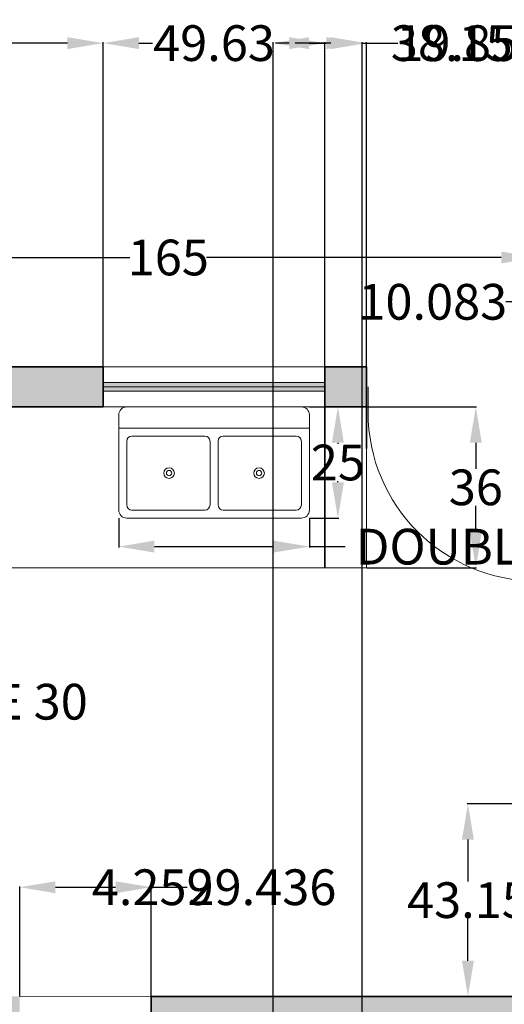
# Model space of a CAD drawing. Units: inches. Extents: x -52 to 678, y 23 to 685.
# Tile 7 of 11: x 141 to 249, y 334 to 555. Entities that reach past the tile are written whole.
import ezdxf

# ---------------------------------------------------------------- set-up
doc = ezdxf.new("R2010")
doc.units = ezdxf.units.IN
doc.header["$MEASUREMENT"] = 0
for name, color, linetype, lineweight in [('A-ANNO-DIMS', 2, 'Continuous', 18), ('A-DOOR', 3, 'Continuous', 18), ('A-FLOR-CASE', 8, 'Continuous', 18), ('A-FLOR-FIXT', 9, 'Continuous', 18), ('A-GLAZ', 4, 'Continuous', 18), ('A-WALL', 7, 'Continuous', 35)]:
    doc.layers.add(name, color=color, linetype=linetype, lineweight=lineweight)
doc.layers.add('A-GLAZ-PATT', color=18, linetype='Continuous', lineweight=13, true_color=0x000000)
doc.layers.add('A-WALL-PATT', color=18, linetype='Continuous', lineweight=13, true_color=0x000000)
doc.styles.get("Standard").update_dxf_attribs({"font": 'arial.ttf'})
doc.dimstyles.get("Standard").update_dxf_attribs({"dimtxt": 8, "dimasz": 8, "dimexe": 0.18, "dimexo": 0.0625, "dimgap": 0.09, "dimtad": 0, "dimtih": 1, "dimtoh": 1, "dimdec": 0, "dimzin": 0, "dimdsep": 46, "dimlunit": 3, "dimtxsty": 'Standard', "dimcen": 0.09, "dimadec": 0, "dimazin": 0, "dimtfac": 1, "dimtdec": 0, "dimtofl": 0, "dimtmove": 0, "dimatfit": 3, "dimfxl": 1, "dimtolj": 1, "dimtzin": 0, "dimarcsym": 0})

# ---------------------------------------------------------------- blocks, each defined once
blk = doc.blocks.new('Sink-double - 36 in top')
for p, q in [((-18, -4), (18, -4)), ((-0.75, -18.5), (-0.75, -6.5)), ((0.75, -6.5), (0.75, -18.5))]:
    blk.add_line(p, q)
for points in [[(-16.5, 0), (16.5, 0)], [(-18, -19.5), (-18, -1.5)], [(18, -1.5), (18, -19.5)], [(-15.5, -5.5), (-1.75, -5.5)], [(1.75, -5.5), (15.5, -5.5)], [(-16.5, -18.5), (-16.5, -6.5)], [(16.5, -6.5), (16.5, -18.5)], [(-1.75, -19.5), (-15.5, -19.5)], [(15.5, -19.5), (1.75, -19.5)], [(16.5, -21), (-16.5, -21)]]:
    blk.add_lwpolyline(points)
for centre, radius in [((-8.5, -12.5), 1), ((-8.5, -12.5), 0.5), ((8.5, -12.5), 1), ((8.5, -12.5), 0.5)]:
    blk.add_circle(centre, radius)
for centre, radius, start, end in [((-16.5, -1.5), 1.5, 90, 180), ((16.5, -1.5), 1.5, 0, 90), ((-15.5, -6.5), 1, 90, 180), ((-1.75, -6.5), 1, 0, 90), ((1.75, -6.5), 1, 90, 180), ((15.5, -6.5), 1, 0, 90), ((-15.5, -18.5), 1, 180, 270), ((-1.75, -18.5), 1, 270, 0), ((1.75, -18.5), 1, 180, 270), ((15.5, -18.5), 1, 270, 0), ((-16.5, -19.5), 1.5, 180, 270), ((16.5, -19.5), 1.5, 270, 0)]:
    blk.add_arc(centre, radius, start, end)
blk = doc.blocks.new('*U16')
for p, q in [((-40, 0), (-40, 6)), ((0, 0), (0, 6))]:
    blk.add_line(p, q)
blk.add_lwpolyline([(0, 0), (0, -40), (-1.75, -40), (-1.75, 0)], close=True)
blk.add_arc((0, 0), 40, 180, 270)
blk = doc.blocks.new('*D29')
at = {"layer": 'A-ANNO-DIMS', "color": 0, "lineweight": -2, "transparency": 16777216}
for p, q in [((163.02, 443.19), (163.02, 436.67)), ((205.67, 443.19), (205.67, 436.67)), ((171.02, 436.85), (197.67, 436.85)), ((205.67, 436.85), (213.67, 436.85))]:
    blk.add_line(p, q, dxfattribs=at)
at = {"layer": 'A-ANNO-DIMS', "color": 0, "transparency": 16777216}
for points in [[(171.02, 438.19), (171.02, 435.52), (163.02, 436.85)], [(197.67, 438.19), (197.67, 435.52), (205.67, 436.85)]]:
    blk.add_solid(points, dxfattribs=at)
at = {"layer": 'Defpoints', "color": 0, "transparency": 16777216}
for p in [(163.02, 443.25), (205.67, 443.25), (205.67, 436.85)]:
    blk.add_point(p, dxfattribs=at)
at = {"layer": 'A-ANNO-DIMS', "color": 0, "transparency": 16777216, "insert": (258.41, 436.85), "char_height": 8, "attachment_point": 5}
blk.add_mtext('\\A1;DOUBLE SINK 43', dxfattribs=at)
blk = doc.blocks.new('*D30')
at = {"layer": 'A-ANNO-DIMS', "color": 0, "lineweight": -2, "transparency": 16777216}
for p, q in [((205.73, 468.13), (212.24, 468.13)), ((212.06, 460.13), (212.06, 459.86)), ((212.06, 451.25), (212.06, 451.51)), ((205.73, 443.25), (212.24, 443.25))]:
    blk.add_line(p, q, dxfattribs=at)
at = {"layer": 'A-ANNO-DIMS', "color": 0, "transparency": 16777216}
for points in [[(210.73, 460.13), (213.4, 460.13), (212.06, 468.13)], [(210.73, 451.25), (213.4, 451.25), (212.06, 443.25)]]:
    blk.add_solid(points, dxfattribs=at)
at = {"layer": 'Defpoints', "color": 0, "transparency": 16777216}
for p in [(205.67, 468.13), (212.06, 468.13), (205.67, 443.25)]:
    blk.add_point(p, dxfattribs=at)
at = {"layer": 'A-ANNO-DIMS', "color": 0, "transparency": 16777216, "insert": (212.06, 455.69), "char_height": 8, "attachment_point": 5}
blk.add_mtext('\\A1;25', dxfattribs=at)
blk = doc.blocks.new('*D31')
at = {"layer": 'A-ANNO-DIMS', "color": 0, "lineweight": -2, "transparency": 16777216}
for p, q in [((126.67, 417.13), (131.29, 417.13)), ((131.11, 409.13), (131.11, 406.36)), ((131.11, 395.13), (131.11, 397.9)), ((126.67, 387.13), (131.29, 387.13))]:
    blk.add_line(p, q, dxfattribs=at)
at = {"layer": 'A-ANNO-DIMS', "color": 0, "transparency": 16777216}
for points in [[(129.77, 409.13), (132.44, 409.13), (131.11, 417.13)], [(129.77, 395.13), (132.44, 395.13), (131.11, 387.13)]]:
    blk.add_solid(points, dxfattribs=at)
at = {"layer": 'Defpoints', "color": 0, "transparency": 16777216}
for p in [(126.61, 417.13), (131.11, 417.13), (126.61, 387.13)]:
    blk.add_point(p, dxfattribs=at)
at = {"layer": 'A-ANNO-DIMS', "color": 0, "transparency": 16777216, "insert": (131.11, 402.13), "char_height": 8, "attachment_point": 5}
blk.add_mtext('\\A1;RANGE 30', dxfattribs=at)
blk = doc.blocks.new('*D41')
at = {"layer": 'A-ANNO-DIMS', "color": 0, "lineweight": -2, "transparency": 16777216}
for p, q in [((91.61, 477.19), (91.61, 501.77)), ((99.61, 501.59), (165.52, 501.59)), ((248.61, 501.59), (182.69, 501.59)), ((256.61, 477.19), (256.61, 501.77))]:
    blk.add_line(p, q, dxfattribs=at)
at = {"layer": 'A-ANNO-DIMS', "color": 0, "transparency": 16777216}
for points in [[(99.61, 502.92), (99.61, 500.25), (91.61, 501.59)], [(248.61, 502.92), (248.61, 500.25), (256.61, 501.59)]]:
    blk.add_solid(points, dxfattribs=at)
at = {"layer": 'Defpoints', "color": 0, "transparency": 16777216}
for p in [(256.61, 501.59), (91.61, 477.13), (256.61, 477.13)]:
    blk.add_point(p, dxfattribs=at)
at = {"layer": 'A-ANNO-DIMS', "color": 0, "transparency": 16777216, "insert": (174.11, 501.59), "char_height": 8, "attachment_point": 5}
blk.add_mtext('\\A1;165', dxfattribs=at)
blk = doc.blocks.new('*D61')
at = {"layer": 'A-ANNO-DIMS', "color": 0, "lineweight": -2, "transparency": 16777216}
for p, q in [((210.46, 549.59), (202.46, 549.59)), ((218.46, 477.19), (218.46, 549.77)), ((256.61, 477.19), (256.61, 549.77)), ((264.61, 549.59), (272.61, 549.59))]:
    blk.add_line(p, q, dxfattribs=at)
at = {"layer": 'A-ANNO-DIMS', "color": 0, "transparency": 16777216}
for points in [[(210.46, 550.92), (210.46, 548.25), (218.46, 549.59)], [(264.61, 550.92), (264.61, 548.25), (256.61, 549.59)]]:
    blk.add_solid(points, dxfattribs=at)
at = {"layer": 'Defpoints', "color": 0, "transparency": 16777216}
for p in [(256.61, 549.59), (218.46, 477.13), (256.61, 477.13)]:
    blk.add_point(p, dxfattribs=at)
at = {"layer": 'A-ANNO-DIMS', "color": 0, "transparency": 16777216, "insert": (237.53, 549.59), "char_height": 8, "attachment_point": 5}
blk.add_mtext('\\A1;38.15', dxfattribs=at)
blk = doc.blocks.new('*D62')
at = {"layer": 'A-ANNO-DIMS', "color": 0, "lineweight": -2, "transparency": 16777216}
for p, q in [((159.53, 477.19), (159.53, 549.77)), ((167.53, 549.59), (170.6, 549.59)), ((201.16, 549.59), (198.09, 549.59)), ((209.16, 477.19), (209.16, 549.77))]:
    blk.add_line(p, q, dxfattribs=at)
at = {"layer": 'A-ANNO-DIMS', "color": 0, "transparency": 16777216}
for points in [[(167.53, 550.92), (167.53, 548.25), (159.53, 549.59)], [(201.16, 550.92), (201.16, 548.25), (209.16, 549.59)]]:
    blk.add_solid(points, dxfattribs=at)
at = {"layer": 'Defpoints', "color": 0, "transparency": 16777216}
for p in [(209.16, 549.59), (159.53, 477.13), (209.16, 477.13)]:
    blk.add_point(p, dxfattribs=at)
at = {"layer": 'A-ANNO-DIMS', "color": 0, "transparency": 16777216, "insert": (184.34, 549.59), "char_height": 8, "attachment_point": 5}
blk.add_mtext('\\A1;49.63', dxfattribs=at)
blk = doc.blocks.new('*D63')
at = {"layer": 'A-ANNO-DIMS', "color": 0, "lineweight": -2, "transparency": 16777216}
for p, q in [((91.61, 477.19), (91.61, 549.77)), ((99.61, 549.59), (112, 549.59)), ((151.53, 549.59), (139.14, 549.59)), ((159.53, 477.19), (159.53, 549.77))]:
    blk.add_line(p, q, dxfattribs=at)
at = {"layer": 'A-ANNO-DIMS', "color": 0, "transparency": 16777216}
for points in [[(99.61, 550.92), (99.61, 548.25), (91.61, 549.59)], [(151.53, 550.92), (151.53, 548.25), (159.53, 549.59)]]:
    blk.add_solid(points, dxfattribs=at)
at = {"layer": 'Defpoints', "color": 0, "transparency": 16777216}
for p in [(159.53, 549.59), (91.61, 477.13), (159.53, 477.13)]:
    blk.add_point(p, dxfattribs=at)
at = {"layer": 'A-ANNO-DIMS', "color": 0, "transparency": 16777216, "insert": (125.57, 549.59), "char_height": 8, "attachment_point": 5}
blk.add_mtext('\\A1;67.92', dxfattribs=at)
blk = doc.blocks.new('*D65')
at = {"layer": 'A-ANNO-DIMS', "color": 0, "lineweight": -2, "transparency": 16777216}
for p, q in [((265.61, 516.06), (265.61, 491.49)), ((275.69, 516.06), (275.69, 491.49)), ((257.61, 491.67), (249.61, 491.67)), ((283.69, 491.67), (291.69, 491.67))]:
    blk.add_line(p, q, dxfattribs=at)
at = {"layer": 'A-ANNO-DIMS', "color": 0, "transparency": 16777216}
for points in [[(257.61, 493), (257.61, 490.33), (265.61, 491.67)], [(283.69, 493), (283.69, 490.33), (275.69, 491.67)]]:
    blk.add_solid(points, dxfattribs=at)
at = {"layer": 'Defpoints', "color": 0, "transparency": 16777216}
for p in [(265.61, 516.13), (275.69, 516.13), (265.61, 491.67)]:
    blk.add_point(p, dxfattribs=at)
at = {"layer": 'A-ANNO-DIMS', "color": 0, "transparency": 16777216, "insert": (233.29, 491.67), "char_height": 8, "attachment_point": 5}
blk.add_mtext('\\A1;10.083', dxfattribs=at)
blk = doc.blocks.new('*D70')
at = {"layer": 'A-ANNO-DIMS', "color": 0, "lineweight": -2, "transparency": 16777216}
for p, q in [((140.86, 336.19), (140.86, 360.77)), ((148.86, 360.59), (162.3, 360.59)), ((170.3, 336.19), (170.3, 360.77)), ((170.3, 360.59), (178.3, 360.59))]:
    blk.add_line(p, q, dxfattribs=at)
at = {"layer": 'A-ANNO-DIMS', "color": 0, "transparency": 16777216}
for points in [[(148.86, 361.92), (148.86, 359.25), (140.86, 360.59)], [(162.3, 361.92), (162.3, 359.25), (170.3, 360.59)]]:
    blk.add_solid(points, dxfattribs=at)
at = {"layer": 'Defpoints', "color": 0, "transparency": 16777216}
for p in [(170.3, 360.59), (140.86, 336.13), (170.3, 336.13)]:
    blk.add_point(p, dxfattribs=at)
at = {"layer": 'A-ANNO-DIMS', "color": 0, "transparency": 16777216, "insert": (195.06, 360.59), "char_height": 8, "attachment_point": 5}
blk.add_mtext('\\A1;29.436', dxfattribs=at)
blk = doc.blocks.new('*D72')
at = {"layer": 'A-ANNO-DIMS', "color": 0, "lineweight": -2, "transparency": 16777216}
for p, q in [((128.61, 360.59), (120.61, 360.59)), ((136.61, 336.19), (136.61, 360.77)), ((140.86, 336.19), (140.86, 360.77)), ((148.86, 360.59), (156.86, 360.59))]:
    blk.add_line(p, q, dxfattribs=at)
at = {"layer": 'A-ANNO-DIMS', "color": 0, "transparency": 16777216}
for points in [[(128.61, 361.92), (128.61, 359.25), (136.61, 360.59)], [(148.86, 361.92), (148.86, 359.25), (140.86, 360.59)]]:
    blk.add_solid(points, dxfattribs=at)
at = {"layer": 'Defpoints', "color": 0, "transparency": 16777216}
for p in [(140.86, 360.59), (136.61, 336.13), (140.86, 336.13)]:
    blk.add_point(p, dxfattribs=at)
at = {"layer": 'A-ANNO-DIMS', "color": 0, "transparency": 16777216, "insert": (170.62, 360.59), "char_height": 8, "attachment_point": 5}
blk.add_mtext('\\A1;4.259', dxfattribs=at)
blk = doc.blocks.new('*D73')
at = {"layer": 'A-ANNO-DIMS', "color": 0, "lineweight": -2, "transparency": 16777216}
for p, q in [((218.52, 468.13), (243.1, 468.13)), ((242.92, 460.13), (242.92, 454.3)), ((242.92, 440.13), (242.92, 445.95)), ((218.52, 432.13), (243.1, 432.13))]:
    blk.add_line(p, q, dxfattribs=at)
at = {"layer": 'A-ANNO-DIMS', "color": 0, "transparency": 16777216}
for points in [[(241.58, 460.13), (244.25, 460.13), (242.92, 468.13)], [(241.58, 440.13), (244.25, 440.13), (242.92, 432.13)]]:
    blk.add_solid(points, dxfattribs=at)
at = {"layer": 'Defpoints', "color": 0, "transparency": 16777216}
for p in [(218.46, 468.13), (218.46, 432.13), (242.92, 432.13)]:
    blk.add_point(p, dxfattribs=at)
at = {"layer": 'A-ANNO-DIMS', "color": 0, "transparency": 16777216, "insert": (242.92, 450.13), "char_height": 8, "attachment_point": 5}
blk.add_mtext('\\A1;36', dxfattribs=at)
blk = doc.blocks.new('*D84')
at = {"layer": 'A-ANNO-DIMS', "color": 0, "lineweight": -2, "transparency": 16777216}
for p, q in [((265.54, 379.27), (240.97, 379.27)), ((241.15, 371.27), (241.15, 361.88)), ((241.15, 344.13), (241.15, 353.52)), ((265.54, 336.13), (240.97, 336.13))]:
    blk.add_line(p, q, dxfattribs=at)
at = {"layer": 'A-ANNO-DIMS', "color": 0, "transparency": 16777216}
for points in [[(239.81, 371.27), (242.48, 371.27), (241.15, 379.27)], [(239.81, 344.13), (242.48, 344.13), (241.15, 336.13)]]:
    blk.add_solid(points, dxfattribs=at)
at = {"layer": 'Defpoints', "color": 0, "transparency": 16777216}
for p in [(241.15, 379.27), (265.61, 379.27), (265.61, 336.13)]:
    blk.add_point(p, dxfattribs=at)
at = {"layer": 'A-ANNO-DIMS', "color": 0, "transparency": 16777216, "insert": (241.15, 357.7), "char_height": 8, "attachment_point": 5}
blk.add_mtext('\\A1;43.15', dxfattribs=at)
blk = doc.blocks.new('*D103')
at = {"layer": 'A-ANNO-DIMS', "color": 0, "lineweight": -2, "transparency": 16777216}
for p, q in [((197.61, 266.24), (197.61, 549.77)), ((205.61, 549.59), (209.46, 549.59)), ((217.46, 271.45), (217.46, 549.77)), ((217.46, 549.59), (225.46, 549.59))]:
    blk.add_line(p, q, dxfattribs=at)
at = {"layer": 'A-ANNO-DIMS', "color": 0, "transparency": 16777216}
for points in [[(205.61, 550.92), (205.61, 548.25), (197.61, 549.59)], [(209.46, 550.92), (209.46, 548.25), (217.46, 549.59)]]:
    blk.add_solid(points, dxfattribs=at)
at = {"layer": 'Defpoints', "color": 0, "transparency": 16777216}
for p in [(217.46, 549.59), (217.46, 271.39), (197.61, 266.17)]:
    blk.add_point(p, dxfattribs=at)
at = {"layer": 'A-ANNO-DIMS', "color": 0, "transparency": 16777216, "insert": (241.78, 549.59), "char_height": 8, "attachment_point": 5}
blk.add_mtext('\\A1;19.856', dxfattribs=at)

msp = doc.modelspace()

# ---------------------------------------------------------------- hatches: boundary and pattern name
at = {"layer": 'A-GLAZ-PATT'}
h = msp.add_hatch(color=256, dxfattribs=at)
h.dxf.hatch_style = 1
h.paths.add_polyline_path([(159.5302, 473.6267), (159.5302, 472.6267), (209.1582, 472.6267), (209.1582, 473.6267)])
h = msp.add_hatch(color=256, dxfattribs=at)
h.dxf.hatch_style = 1
h.paths.add_polyline_path([(159.5302, 472.6267), (159.5302, 471.6267), (209.1582, 471.6267), (209.1582, 472.6267)])
at = {"layer": 'A-WALL-PATT'}
h = msp.add_hatch(color=256, dxfattribs=at)
h.dxf.hatch_style = 1
h.paths.add_polyline_path([(100.6053, 336.1267), (100.6053, 468.1267), (159.5302, 468.1267), (159.5302, 477.1267), (91.6053, 477.1267), (91.6053, 327.1267), (140.8548, 327.1267), (140.8548, 336.1267), (137.7032, 336.1267)])
h = msp.add_hatch(color=256, dxfattribs=at)
h.dxf.hatch_style = 1
h.paths.add_polyline_path([(218.4552, 477.1267), (209.1582, 477.1267), (209.1582, 468.1267), (218.4552, 468.1267)])
h = msp.add_hatch(color=256, dxfattribs=at)
h.dxf.hatch_style = 1
h.paths.add_polyline_path([(265.6053, 327.1267), (265.6053, 336.1267), (170.301, 336.1267), (170.301, 327.1267)])

# ---------------------------------------------------------------- linework, layer by layer
at = {"layer": 'A-FLOR-CASE'}
for p, q in [((218.4552, 468.1267), (218.4552, 432.1267)), ((218.4552, 432.1267), (136.6053, 432.1267))]:
    msp.add_line(p, q, dxfattribs=at)
at = {"layer": 'A-GLAZ'}
for p, q in [((159.5302, 477.1267), (209.1582, 477.1267)), ((159.5302, 473.6267), (209.1582, 473.6267)), ((159.5302, 472.6267), (209.1582, 472.6267)), ((159.5302, 471.6267), (209.1582, 471.6267)), ((159.5302, 468.1267), (209.1582, 468.1267)), ((140.8646, 336.1267), (170.3108, 336.0613))]:
    msp.add_line(p, q, dxfattribs=at)
at = {"layer": 'A-WALL'}
for p, q in [((91.6053, 477.1267), (159.5302, 477.1267)), ((159.5302, 477.1267), (159.5302, 468.1267)), ((209.1582, 477.1267), (209.1582, 432.1267)), ((209.1582, 477.1267), (218.4552, 477.1267)), ((218.4552, 458.8319), (218.4552, 477.1267)), ((100.6053, 468.1267), (159.5302, 468.1267)), ((209.1582, 468.1267), (218.4552, 468.1267)), ((170.301, 327.1267), (170.301, 336.1267)), ((170.301, 336.1267), (265.6053, 336.1267))]:
    msp.add_line(p, q, dxfattribs=at)

# ---------------------------------------------------------------- block references
at = {"layer": 'A-DOOR', "xscale": 0.9449538553603543, "yscale": 0.9449538553603543, "zscale": 0.9449538553603543}
msp.add_blockref('*U16', (256.6053, 466.957), dxfattribs=at)
at = {"layer": 'A-FLOR-FIXT', "xscale": 1.184572414652458, "yscale": 1.184572414652458, "zscale": 1.184572414652458}
msp.add_blockref('Sink-double - 36 in top', (184.3442, 468.1267), dxfattribs=at)

# ---------------------------------------------------------------- dimensions: what is measured, and where the dimension line sits
at = {"layer": 'A-ANNO-DIMS'}
for base, p1, p2, override, picture, middle in [((159.5302, 549.5867), (91.6053, 477.1267), (159.5302, 477.1267), {"dimdec": 2, "dimlfac": 1, "dimrnd": 0, "dimzin": 0, "dimdsep": 46, "dimlunit": 2}, '*D63', (125.5677, 549.5867)), ((209.1582, 549.5867), (159.5302, 477.1267), (209.1582, 477.1267), {"dimdec": 2, "dimlfac": 1, "dimrnd": 0, "dimzin": 0, "dimdsep": 46, "dimlunit": 2}, '*D62', (184.3442, 549.5867)), ((217.4609, 549.5867), (197.6053, 266.1726), (217.4609, 271.3879), {"dimdec": 3, "dimlfac": 1, "dimrnd": 0, "dimzin": 0, "dimdsep": 46, "dimlunit": 2}, '*D103', (241.7774, 549.5867)), ((256.6053, 549.5867), (218.4552, 477.1267), (256.6053, 477.1267), {"dimdec": 2, "dimlfac": 1, "dimrnd": 0, "dimzin": 0, "dimdsep": 46, "dimlunit": 2}, '*D61', (237.5302, 549.5867))]:
    dim = msp.add_linear_dim(base=base, p1=p1, p2=p2, dimstyle='Standard', override=override, dxfattribs=at)
    dim.commit()
    dim.dimension.update_dxf_attribs({"geometry": picture, "text_midpoint": middle})
for base, p1, p2, angle, override, picture, middle in [((265.6053, 491.6667), (275.688, 516.1267), (265.6053, 516.1267), 180, {"dimdec": 3, "dimlfac": 1, "dimrnd": 0, "dimzin": 0, "dimdsep": 46, "dimlunit": 2}, '*D65', (233.2861, 491.6667)), ((256.6053, 501.5867), (91.6053, 477.1267), (256.6053, 477.1267), 0, {"dimdec": 0, "dimlfac": 1, "dimrnd": 0, "dimzin": 0, "dimdsep": 46, "dimlunit": 2}, '*D41', (174.1053, 501.5867)), ((212.0632, 468.1267), (205.6665, 443.2507), (205.6665, 468.1267), 90, {"dimdec": 0, "dimlfac": 1, "dimrnd": 0, "dimzin": 0, "dimdsep": 46, "dimlunit": 2}, '*D30', (212.0632, 455.6887)), ((242.9152, 432.1267), (218.4552, 468.1267), (218.4552, 432.1267), 270, {"dimdec": 0, "dimlfac": 1, "dimrnd": 0, "dimzin": 0, "dimdsep": 46, "dimlunit": 2}, '*D73', (242.9152, 450.1267)), ((241.1453, 379.2738), (265.6053, 336.1267), (265.6053, 379.2738), 90, {"dimdec": 2, "dimlfac": 1, "dimrnd": 0, "dimzin": 0, "dimdsep": 46, "dimlunit": 2}, '*D84', (241.1453, 357.7003)), ((140.8647, 360.5867), (136.6053, 336.1267), (140.8646, 336.1267), 359.999705, {"dimdec": 3, "dimlfac": 1, "dimrnd": 0, "dimzin": 0, "dimdsep": 46, "dimlunit": 2}, '*D72', (170.6219, 360.5866)), ((170.301, 360.5867), (140.8646, 336.1267), (170.301, 336.1267), 0.000043, {"dimdec": 3, "dimlfac": 1, "dimrnd": 0, "dimzin": 0, "dimdsep": 46, "dimlunit": 2}, '*D70', (195.0622, 360.5867))]:
    dim = msp.add_linear_dim(base=base, p1=p1, p2=p2, angle=angle, dimstyle='Standard', override=override, dxfattribs=at)
    dim.commit()
    dim.dimension.update_dxf_attribs({"geometry": picture, "text_midpoint": middle})
dim = msp.add_linear_dim(base=(205.6665, 436.854), p1=(163.0219, 443.2507), p2=(205.6665, 443.2507), text='DOUBLE SINK <>', dimstyle='Standard', override={"dimdec": 0, "dimlfac": 1, "dimrnd": 0, "dimzin": 0, "dimdsep": 46, "dimlunit": 2}, dxfattribs=at)
dim.commit()
dim.dimension.update_dxf_attribs({"geometry": '*D29', "text_midpoint": (258.4141, 436.854)})
dim = msp.add_linear_dim(base=(131.1053, 417.1267), p1=(126.6053, 387.1267), p2=(126.6053, 417.1267), angle=90, text='RANGE <>', dimstyle='Standard', override={"dimdec": 0, "dimlfac": 1, "dimrnd": 0, "dimzin": 0, "dimdsep": 46, "dimlunit": 2}, dxfattribs=at)
dim.commit()
dim.dimension.update_dxf_attribs({"geometry": '*D31', "text_midpoint": (131.1053, 402.1267)})

doc.saveas('drawing.dxf')
